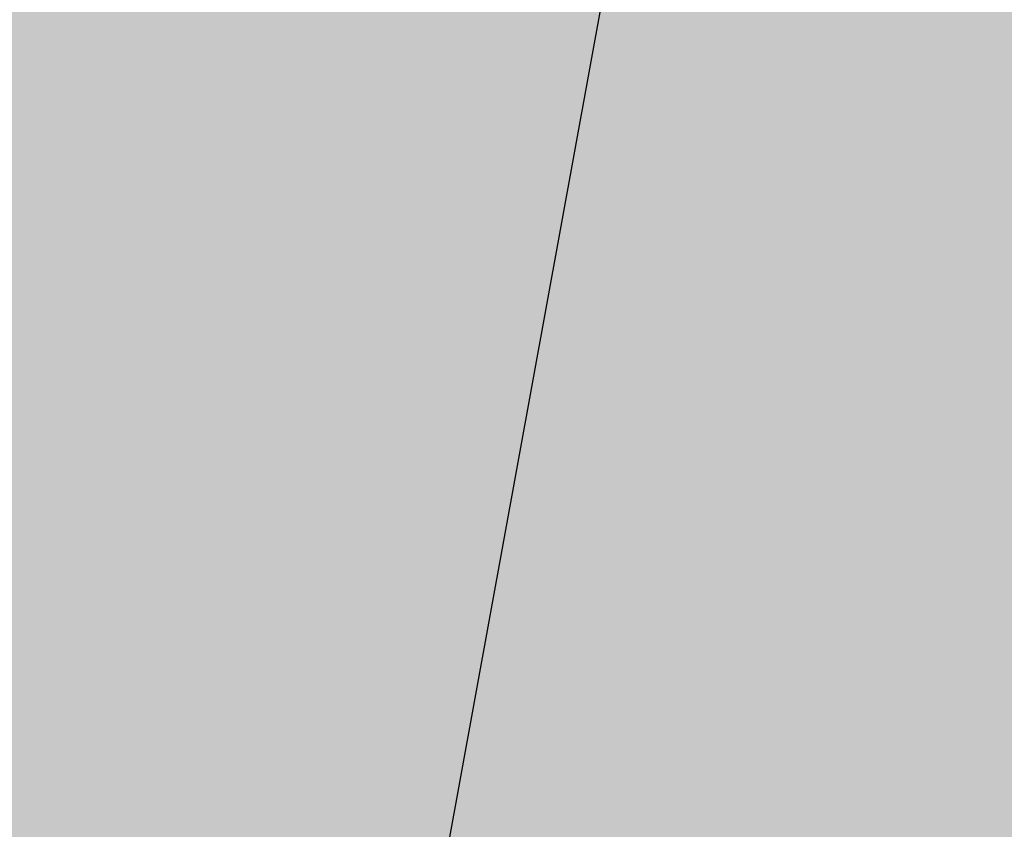
# Model space of a CAD drawing. Units: feet. Extents: x 3168 to 4724, y 827 to 1477.
# Tile 226 of 256: x 3379.08 to 3386.684, y 1087.401 to 1093.654. Entities that reach past the tile are written whole.
import ezdxf

# ---------------------------------------------------------------- set-up
doc = ezdxf.new("R2010")
doc.units = ezdxf.units.FT
doc.layers.add('A-ELEV-PATT', color=8, linetype='Continuous', lineweight=13)
doc.layers.add('C-TOPO', color=3, linetype='Continuous', lineweight=25)

msp = doc.modelspace()

# ---------------------------------------------------------------- hatches: boundary and pattern name
at = {"layer": 'A-ELEV-PATT'}
h = msp.add_hatch(color=256, dxfattribs=at)
h.dxf.hatch_style = 1
edge = h.paths.add_edge_path()
edge.add_ellipse((3552.9058, 979.2201), major_axis=(36.7449, 0), ratio=0.4848485, start_angle=0, end_angle=360)
edge = h.paths.add_edge_path()
edge.add_ellipse((3559.8916, 929.2523), major_axis=(36.7449, 0), ratio=0.4848485, start_angle=0, end_angle=360)
edge = h.paths.add_edge_path()
edge.add_line((3299.3168, 1198.6061), (3479.9167, 1198.6061))
edge.add_line((3479.9167, 1198.6061), (3479.9167, 1209.8686))
edge.add_spline(control_points=[(3479.9167, 1209.8686), (3464.3012, 1209.8686), (3448.6856, 1209.8686), (3410.9491, 1209.8686), (3388.8282, 1209.8686), (3355.6469, 1209.8686), (3344.5864, 1209.8686), (3327.9957, 1209.8686), (3322.4655, 1209.8686), (3314.1702, 1209.8686), (3311.4051, 1209.8686), (3307.2574, 1209.8686), (3305.8748, 1209.8686), (3303.801, 1209.8686), (3303.1097, 1209.8686), (3302.0728, 1209.8686), (3301.7272, 1209.8686), (3301.2087, 1209.8686), (3301.0359, 1209.8686), (3300.7767, 1209.8686), (3300.6903, 1209.8686), (3300.5606, 1209.8686), (3300.5174, 1209.8686), (3300.4526, 1209.8686), (3300.431, 1209.8686), (3300.3986, 1209.8686), (3300.3878, 1209.8686), (3300.3662, 1209.8686), (3300.3457, 1209.8686), (3300.3455, 1209.8686), (3300.3455, 1209.8686), (3300.3433, 1209.8686), (3300.3411, 1209.8686), (3300.3379, 1209.8686), (3300.3368, 1209.8686), (3300.3339, 1209.8686), (3300.3321, 1209.8686), (3300.3255, 1209.8686), (3300.3207, 1209.8686), (3300.3109, 1209.8686), (3300.306, 1209.8686), (3300.2905, 1209.8686), (3300.28, 1209.8686), (3300.2324, 1209.8688), (3300.1953, 1209.869), (3299.9511, 1209.8706), (3299.7448, 1209.8743), (3299.4368, 1209.8833), (3299.3344, 1209.8868), (3299.1811, 1209.8929), (3299.13, 1209.8951), (3298.6522, 1209.9168), (3298.2295, 1209.9457), (3297.6016, 1210.0024), (3297.3934, 1210.0235), (3297.0827, 1210.0583), (3296.9793, 1210.0705), (3296.293, 1210.1549), (3295.7181, 1210.2434), (3294.8687, 1210.3989), (3294.5877, 1210.4545), (3294.1693, 1210.5433), (3294.0304, 1210.5739), (3291.7071, 1211.1012), (3289.6536, 1211.8134), (3285.7763, 1213.564), (3283.9514, 1214.6035), (3280.5122, 1216.9801), (3278.8972, 1218.3176), (3276.3799, 1220.8295), (3275.416, 1221.9177), (3274.0393, 1223.7077), (3273.581, 1224.3495), (3273.1432, 1225.0163)], knot_values=[39.119033, 39.119033, 39.119033, 39.119033, 39.286353, 39.286353, 39.523379, 39.523379, 39.641892, 39.641892, 39.701148, 39.701148, 39.730777, 39.730777, 39.745591, 39.745591, 39.752998, 39.752998, 39.756701, 39.756701, 39.758553, 39.758553, 39.759479, 39.759479, 39.759942, 39.759942, 39.760173, 39.760173, 39.760289, 39.760289, 39.760405, 39.760405, 39.760463, 39.760463, 39.763389, 39.763389, 39.764851, 39.764851, 39.767304, 39.767304, 39.773825, 39.773825, 39.78057, 39.78057, 39.79477, 39.79477, 39.845194, 39.845194, 40.126715, 40.126715, 40.267476, 40.267476, 40.337856, 40.337856, 40.927023, 40.927023, 41.221606, 41.221606, 41.368898, 41.368898, 42.202622, 42.202622, 42.619485, 42.619485, 42.827916, 42.827916, 46.118323, 46.118323, 49.408731, 49.408731, 52.699139, 52.699139, 54.927489, 54.927489, 56.104228, 56.104228, 56.104228, 56.104228], weights=[1, 1, 1, 1, 1, 1, 1, 1, 1, 1, 1, 1, 1, 1, 1, 1, 1, 1, 1, 1, 1, 1, 1, 1, 1, 1, 1, 1, 1, 1, 1, 1, 1, 1, 1, 1, 1, 1, 1, 1, 1, 1, 1, 1, 1, 1, 1, 1, 1, 1, 1, 1, 1, 1, 1, 1, 1, 1, 1, 1, 1, 1, 1, 1, 1, 1, 1, 1, 1, 1, 1, 1, 1, 1], degree=3, periodic=0)
edge.add_line((3273.1432, 1225.0163), (3273.1432, 1099.0163))
edge.add_line((3273.1432, 1099.0163), (3299.3168, 1099.0163))
edge.add_line((3299.3168, 1099.0163), (3299.3168, 1198.6061))
edge = h.paths.add_edge_path()
edge.add_line((3304.7584, 1324.1581), (3479.9167, 1324.1581))
edge.add_line((3479.9167, 1324.1581), (3479.9167, 1335.7146))
edge.add_line((3479.9167, 1335.7146), (3269.1616, 1335.7146))
edge.add_spline(control_points=[(3269.1616, 1335.7146), (3264.0242, 1335.7146), (3258.3641, 1328.9582), (3259.2643, 1323.9003)], knot_values=[0, 0, 0, 0, 15.412191, 15.412191, 15.412191, 15.412191], degree=3, periodic=0)
edge.add_line((3259.2643, 1323.9003), (3265.5168, 1288.7691))
edge.add_line((3265.5168, 1288.7691), (3275.2651, 1261.5456))
edge.add_line((3275.2651, 1261.5456), (3304.7584, 1261.5456))
edge.add_line((3304.7584, 1261.5456), (3304.7584, 1324.1581))
h = msp.add_hatch(color=256, dxfattribs=at)
h.dxf.hatch_style = 1
h.paths.add_polyline_path([(3384.5252, 1099.0163), (3335.0292, 1099.0163), (3299.3168, 1099.0163), (3273.1432, 1099.0163), (3217.5654, 1099.0163), (3168.0693, 827.1163), (3335.0292, 827.1163)])
h = msp.add_hatch(color=256, dxfattribs=at)
h.dxf.hatch_style = 1
h.paths.add_polyline_path([(3845.3757, 1099.0163), (3706.2884, 1099.0163), (3715.6187, 1081.3955), (3715.6187, 1052.3102), (3792.0552, 907.9557), (3463.2221, 903.6425), (3462.8992, 928.2574, 0.540152), (3462.8992, 1014.0826), (3621.8987, 1014.0826), (3601.657, 1052.3102), (3601.657, 1081.3955), (3592.3267, 1099.0163), (3384.5252, 1099.0163), (3335.0292, 827.1163), (3845.3757, 827.1163)])

# ---------------------------------------------------------------- linework, layer by layer
at = {"layer": 'C-TOPO'}
msp.add_line((3384.5252, 1099.0163), (3335.0292, 827.1163), dxfattribs=at)
msp.add_lwpolyline([(3384.5252, 1099.0163), (3335.0292, 827.1163), (3845.3757, 827.1163), (3845.3757, 1099.0163), (3335.0292, 1099.0163)], dxfattribs=at)

doc.saveas('drawing.dxf')
